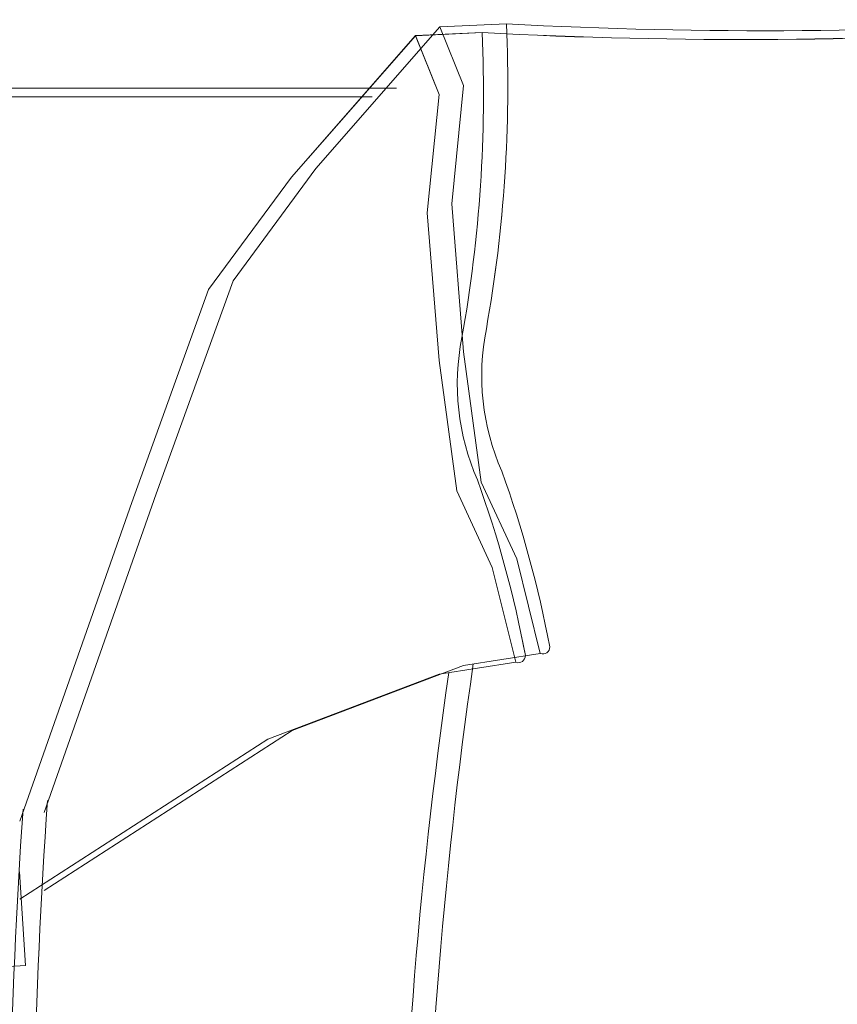
# Model space of a CAD drawing. Units: inches. Extents: x 1901 to 2863, y 888 to 2433.
# Tile 59 of 91: x 2049 to 2073, y 2161 to 2190. Entities that reach past the tile are written whole.
import ezdxf

# ---------------------------------------------------------------- set-up
doc = ezdxf.new("R2010")
doc.units = ezdxf.units.IN
doc.layers.add('A-FURN', color=8, linetype='Continuous', lineweight=18)

# ---------------------------------------------------------------- blocks, each defined once
blk = doc.blocks.new('BED-DOUBLE')
for p, q in [((33.854, 59.666), (31.896, 59.577, 4.346)), ((33.854, 59.666), (31.896, 59.577, 4.346)), ((31.896, 59.577), (28.246, 55.417)), ((31.896, 59.577), (28.246, 55.417)), ((33.137, 59.41), (31.178, 59.321, 4.346)), ((33.137, 59.41), (31.178, 59.32, 4.346)), ((32.591, 57.851), (31.896, 59.577)), ((32.591, 57.851), (31.896, 59.577)), ((31.178, 59.321), (27.529, 55.161)), ((31.178, 59.32), (27.529, 55.16)), ((31.873, 57.595), (31.178, 59.321)), ((31.873, 57.595), (31.178, 59.32)), ((0.744, 57.778), (30.62, 57.778)), ((0.744, 57.778), (30.62, 57.778)), ((31.525, 54.117), (31.873, 57.595)), ((31.525, 54.117), (31.873, 57.595)), ((32.243, 54.374), (32.591, 57.851)), ((32.243, 54.373), (32.591, 57.851)), ((28.246, 55.417), (25.814, 52.113)), ((28.246, 55.417), (25.814, 52.113)), ((27.529, 55.161), (25.096, 51.857)), ((27.529, 55.16), (25.096, 51.856)), ((32.591, 50.027), (32.243, 54.374)), ((32.591, 50.026), (32.243, 54.373)), ((31.873, 49.77), (31.525, 54.117)), ((31.873, 49.77), (31.525, 54.117)), ((25.814, 52.113), (23.554, 45.853)), ((25.814, 52.113), (23.554, 45.853)), ((25.096, 51.857), (22.837, 45.597)), ((25.096, 51.856), (22.837, 45.597)), ((33.112, 46.201), (32.591, 50.027)), ((33.112, 46.201), (32.591, 50.026)), ((32.394, 45.945), (31.873, 49.77)), ((32.394, 45.944), (31.873, 49.77)), ((34.155, 43.941), (33.112, 46.201)), ((34.155, 43.94), (33.112, 46.201)), ((23.554, 45.853), (20.261, 36.492)), ((23.554, 45.853), (20.261, 36.491)), ((33.437, 43.684), (32.394, 45.945)), ((33.437, 43.684), (32.394, 45.944)), ((22.837, 45.597), (19.543, 36.235)), ((22.837, 45.597), (19.543, 36.235)), ((34.85, 41.158), (34.155, 43.941)), ((34.85, 41.158), (34.155, 43.94)), ((34.132, 40.902), (33.437, 43.684)), ((34.132, 40.902), (33.437, 43.684)), ((32.591, 40.811), (34.85, 41.158)), ((32.591, 40.81), (34.85, 41.158)), ((27.551, 38.898), (32.591, 40.811)), ((27.551, 38.898), (32.591, 40.81)), ((31.873, 40.554), (34.132, 40.902)), ((31.873, 40.554), (34.132, 40.902)), ((26.834, 38.642), (31.873, 40.554)), ((26.834, 38.641), (31.873, 40.554)), ((20.261, 34.194), (27.551, 38.898)), ((20.261, 34.193), (27.551, 38.898)), ((19.543, 33.937), (26.834, 38.642)), ((19.543, 33.937), (26.834, 38.641)), ((19.71, 31.991), (19.538, 34.745)), ((19.71, 31.991), (19.538, 34.745)), ((16.706, 31.803), (19.71, 31.991)), ((16.706, 31.803), (19.71, 31.991))]:
    blk.add_line(p, q)
for centre, radius, start, end in [((-6.729, 57.848), 40.624, 349.8763, 2.5657), ((-6.729, 57.847), 40.624, 349.8763, 2.5657), ((41.517, 204.859), 145.395, 266.97912, 273.83645), ((41.517, 204.859), 145.395, 266.97912, 273.83645), ((-7.447, 57.591), 40.624, 349.8763, 2.5657), ((-7.447, 57.591), 40.624, 349.8763, 2.5657), ((40.799, 204.603), 145.395, 266.97912, 273.83645), ((40.799, 204.602), 145.395, 266.97912, 273.83645), ((40.115, 49.333), 6.988, 168.6608, 203.7384), ((40.115, 49.333), 6.988, 168.6608, 203.7384), ((39.397, 49.077), 6.988, 168.6608, 203.7384), ((39.397, 49.076), 6.988, 168.6608, 203.7384), ((2.408, 35.198), 33.294, 10.6617, 19.8806), ((2.408, 35.198), 33.294, 10.6617, 19.8806), ((1.69, 34.942), 33.294, 10.6617, 19.8806), ((1.69, 34.941), 33.294, 10.6617, 19.8806), ((34.202, 41.097), 0.207, 250.2464, 1.1377), ((34.202, 41.097), 0.207, 250.2464, 1.1377), ((34.92, 41.353), 0.207, 250.2464, 1.1377), ((34.92, 41.353), 0.207, 250.2464, 1.1377), ((176.248, 20.155), 144.857, 171.78449, 186.90062), ((176.248, 20.155), 144.857, 171.78449, 186.90062), ((175.53, 19.899), 144.857, 171.78449, 186.90062), ((175.53, 19.899), 144.857, 171.78449, 186.90062), ((205.143, 24.201), 185.219, 176.08655, 186.78213), ((205.143, 24.2), 185.219, 176.08655, 186.78213), ((204.426, 23.944), 185.219, 176.08655, 186.78213), ((204.426, 23.944), 185.219, 176.08655, 186.78213)]:
    blk.add_arc(centre, radius, start, end)

msp = doc.modelspace()

# ---------------------------------------------------------------- linework, layer by layer
at = {"layer": 'A-FURN'}
msp.add_line((2029.426, 2187.522), (2059.302, 2187.522), dxfattribs=at)
msp.add_line((2029.426, 2187.522), (2059.302, 2187.522), dxfattribs=at)

# ---------------------------------------------------------------- block references
msp.add_blockref('BED-DOUBLE', (2029.4, 2130), dxfattribs=at)

doc.saveas('drawing.dxf')
